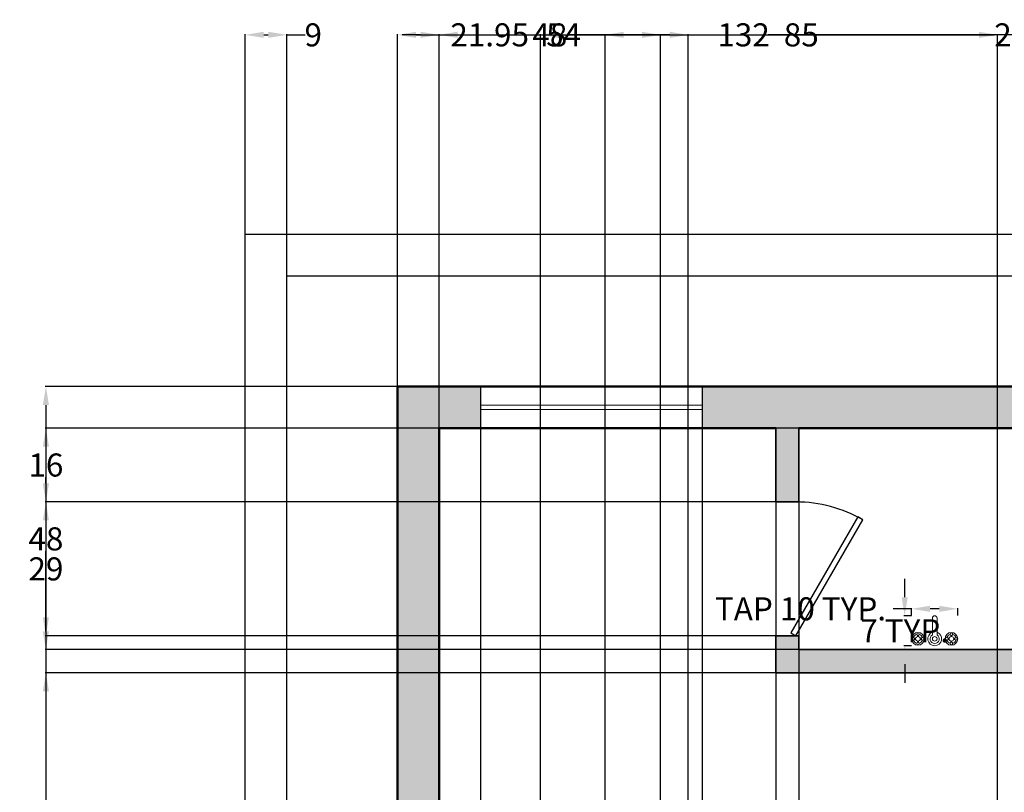
# Model space of a CAD drawing. Units: inches. Extents: x 882 to 1363, y 890 to 1847.
# Tile 8 of 9: x 901 to 1114, y 1680 to 1847. Entities that reach past the tile are written whole.
import ezdxf

# ---------------------------------------------------------------- set-up
doc = ezdxf.new("R2010")
doc.units = ezdxf.units.IN
doc.header["$MEASUREMENT"] = 0
for name, color, linetype, lineweight in [('A-ANNO-DIMS', 2, 'Continuous', 18), ('C-PROP', 7, 'Continuous', 25), ('doors', 3, 'Continuous', 25), ('inner wall', 50, 'Continuous', 35), ('outer wall', 40, 'Continuous', 50), ('sanitary', 231, 'Continuous', 18), ('windows', 226, 'Continuous', 18)]:
    doc.layers.add(name, color=color, linetype=linetype, lineweight=lineweight)
doc.layers.add('A-WALL-PATT', color=251, linetype='Continuous', lineweight=13, true_color=0x636466)
doc.styles.get("Standard").update_dxf_attribs({"font": 'arial.ttf'})
doc.dimstyles.get("Standard").update_dxf_attribs({"dimtxt": 5, "dimasz": 4, "dimexe": 0.18, "dimexo": 0.0625, "dimgap": 0.09, "dimtad": 0, "dimtih": 1, "dimtoh": 1, "dimdec": 1, "dimzin": 0, "dimdsep": 46, "dimlunit": 3, "dimtxsty": 'Standard', "dimcen": 0.09, "dimadec": 0, "dimazin": 0, "dimtfac": 1, "dimtdec": 1, "dimtofl": 0, "dimtmove": 0, "dimatfit": 3, "dimfxl": 1, "dimtolj": 1, "dimtzin": 0, "dimarcsym": 0})

# ---------------------------------------------------------------- blocks, each defined once
blk = doc.blocks.new('*U4')
for p, q in [((0, 0), (0, -6)), ((-40, 0), (-40, -6))]:
    blk.add_line(p, q)
blk.add_lwpolyline([(0, 0), (-34.64, 20), (-35.52, 18.48), (-0.88, -1.52)], close=True)
blk.add_arc((0, 0), 40, 150, 180)
blk = doc.blocks.new('Faucet - Bathroom top')
for p, q in [((-4.107, 0.125), (-4.375, 0.125)), ((-3.75, 0.4788), (-3.75, 0.75)), ((-3.5, 0.482), (-3.5, 0.75)), ((-3.1461, 0.125), (-2.875, 0.125)), ((3.143, 0.125), (2.875, 0.125)), ((3.5, 0.4788), (3.5, 0.75)), ((3.75, 0.482), (3.75, 0.75)), ((4.1039, 0.125), (4.375, 0.125)), ((-4.1039, -0.125), (-4.375, -0.125)), ((-3.75, -0.4821), (-3.75, -0.75)), ((-3.5, -0.4789), (-3.5, -0.75)), ((-3.143, -0.125), (-2.875, -0.125)), ((-0.5, -0.8639), (-0.5, -4.5)), ((0.5, -4.5), (0.5, -0.8631)), ((3.1461, -0.125), (2.875, -0.125)), ((3.5, -0.4821), (3.5, -0.75)), ((3.75, -0.4789), (3.75, -0.75)), ((4.107, -0.125), (4.375, -0.125))]:
    blk.add_line(p, q)
for centre, radius in [((-3.625, 0), 1.375), ((-4.625, 0), 0.2795), ((-3.625, 0), 0.5), ((-3.625, 1), 0.2795), ((-2.625, 0), 0.2795), ((0, 0), 0.5), ((3.625, 0), 1.375), ((2.625, 0), 0.2795), ((3.625, 0), 0.5), ((3.625, 1), 0.2795), ((4.625, 0), 0.2795), ((-3.625, -1), 0.2795), ((3.625, -1), 0.2795)]:
    blk.add_circle(centre, radius)
for centre, radius, start, end in [((-3.625, 0), 1, 105.2407, 164.2093), ((-3.625, 0), 1, 16.44125, 74.07887), ((0, 0), 1.5, 289.6514, 250.3603), ((0, 0), 1, 300.3431, 239.7554), ((3.625, 0), 1, 106.12, 164.0884), ((3.625, 0), 1, 16.23422, 73.90469), ((-3.625, 0), 1, 196.2342, 253.9047), ((-3.625, 0), 1, 286.12, 344.0884), ((3.625, 0), 1, 196.4413, 254.0789), ((3.625, 0), 1, 285.2407, 344.2093), ((0, -4.5), 0.5, 180, 0)]:
    blk.add_arc(centre, radius, start, end)
blk = doc.blocks.new('*D21')
at = {"layer": 'A-ANNO-DIMS', "color": 0, "lineweight": -2, "transparency": 16777216}
for p, q in [((1094.25, 1719.59), (1090.25, 1719.59)), ((1094.25, 1718.15), (1094.25, 1719.77)), ((1100.25, 1719.59), (1098.25, 1719.59)), ((1104.25, 1718.15), (1104.25, 1719.77))]:
    blk.add_line(p, q, dxfattribs=at)
at = {"layer": 'A-ANNO-DIMS', "color": 0, "transparency": 16777216}
for points in [[(1098.25, 1720.26), (1098.25, 1718.93), (1094.25, 1719.59)], [(1100.25, 1720.26), (1100.25, 1718.93), (1104.25, 1719.59)]]:
    blk.add_solid(points, dxfattribs=at)
at = {"layer": 'Defpoints', "color": 0, "transparency": 16777216}
for p in [(1094.25, 1719.59), (1094.25, 1718.09), (1104.25, 1718.09)]:
    blk.add_point(p, dxfattribs=at)
at = {"layer": 'A-ANNO-DIMS', "color": 0, "transparency": 16777216, "insert": (1070.17, 1719.59), "char_height": 5, "attachment_point": 5}
blk.add_mtext('\\A1;TAP 10 TYP.', dxfattribs=at)
blk = doc.blocks.new('*D22')
at = {"layer": 'A-ANNO-DIMS', "color": 0, "lineweight": -2, "transparency": 16777216}
for p, q in [((1092.75, 1722.09), (1092.75, 1726.09)), ((1094.19, 1718.09), (1092.57, 1718.09)), ((1094.19, 1711.59), (1092.57, 1711.59)), ((1092.75, 1707.59), (1092.75, 1703.59))]:
    blk.add_line(p, q, dxfattribs=at)
at = {"layer": 'A-ANNO-DIMS', "color": 0, "transparency": 16777216}
for points in [[(1092.09, 1722.09), (1093.42, 1722.09), (1092.75, 1718.09)], [(1092.09, 1707.59), (1093.42, 1707.59), (1092.75, 1711.59)]]:
    blk.add_solid(points, dxfattribs=at)
at = {"layer": 'Defpoints', "color": 0, "transparency": 16777216}
for p in [(1094.25, 1718.09), (1092.75, 1711.59), (1094.25, 1711.59)]:
    blk.add_point(p, dxfattribs=at)
at = {"layer": 'A-ANNO-DIMS', "color": 0, "transparency": 16777216, "insert": (1092.75, 1714.84), "char_height": 5, "attachment_point": 5}
blk.add_mtext('\\A1;7 TYP.', dxfattribs=at)
blk = doc.blocks.new('*D37')
at = {"layer": 'A-ANNO-DIMS', "color": 0, "lineweight": -2, "transparency": 16777216}
for p, q in [((982.78, 1767.75), (906.46, 1767.75)), ((906.64, 1763.75), (906.64, 1383.34)), ((906.64, 997.75), (906.64, 1378.16)), ((982.78, 993.75), (906.46, 993.75))]:
    blk.add_line(p, q, dxfattribs=at)
at = {"layer": 'A-ANNO-DIMS', "color": 0, "transparency": 16777216}
for points in [[(905.97, 1763.75), (907.3, 1763.75), (906.64, 1767.75)], [(905.97, 997.75), (907.3, 997.75), (906.64, 993.75)]]:
    blk.add_solid(points, dxfattribs=at)
at = {"layer": 'Defpoints', "color": 0, "transparency": 16777216}
for p in [(906.64, 1767.75), (982.84, 1767.75), (982.84, 993.75)]:
    blk.add_point(p, dxfattribs=at)
at = {"layer": 'A-ANNO-DIMS', "color": 0, "transparency": 16777216, "insert": (906.64, 1380.75), "char_height": 5, "attachment_point": 5}
blk.add_mtext('\\A1;774', dxfattribs=at)
blk = doc.blocks.new('*D38')
at = {"layer": 'A-ANNO-DIMS', "color": 0, "lineweight": -2, "transparency": 16777216}
for p, q in [((949.84, 1800.81), (949.84, 1844.13)), ((953.84, 1843.95), (954.84, 1843.95)), ((958.84, 1791.81), (958.84, 1844.13)), ((958.84, 1843.95), (962.84, 1843.95))]:
    blk.add_line(p, q, dxfattribs=at)
at = {"layer": 'A-ANNO-DIMS', "color": 0, "transparency": 16777216}
for points in [[(953.84, 1844.62), (953.84, 1843.29), (949.84, 1843.95)], [(954.84, 1844.62), (954.84, 1843.29), (958.84, 1843.95)]]:
    blk.add_solid(points, dxfattribs=at)
at = {"layer": 'Defpoints', "color": 0, "transparency": 16777216}
for p in [(958.84, 1843.95), (949.84, 1800.75), (958.84, 1791.75)]:
    blk.add_point(p, dxfattribs=at)
at = {"layer": 'A-ANNO-DIMS', "color": 0, "transparency": 16777216, "insert": (964.57, 1843.95), "char_height": 5, "attachment_point": 5}
blk.add_mtext('\\A1;9', dxfattribs=at)
blk = doc.blocks.new('*D39')
at = {"layer": 'A-ANNO-DIMS', "color": 0, "lineweight": -2, "transparency": 16777216}
for p, q in [((982.84, 1767.81), (982.84, 1844.13)), ((986.84, 1843.95), (1112.19, 1843.95)), ((1248.84, 1843.95), (1123.49, 1843.95)), ((1252.84, 1767.81), (1252.84, 1844.13))]:
    blk.add_line(p, q, dxfattribs=at)
at = {"layer": 'A-ANNO-DIMS', "color": 0, "transparency": 16777216}
for points in [[(986.84, 1844.62), (986.84, 1843.29), (982.84, 1843.95)], [(1248.84, 1844.62), (1248.84, 1843.29), (1252.84, 1843.95)]]:
    blk.add_solid(points, dxfattribs=at)
at = {"layer": 'Defpoints', "color": 0, "transparency": 16777216}
for p in [(1252.84, 1843.95), (982.84, 1767.75), (1252.84, 1767.75)]:
    blk.add_point(p, dxfattribs=at)
at = {"layer": 'A-ANNO-DIMS', "color": 0, "transparency": 16777216, "insert": (1117.84, 1843.95), "char_height": 5, "attachment_point": 5}
blk.add_mtext('\\A1;270', dxfattribs=at)
blk = doc.blocks.new('*D40')
at = {"layer": 'A-ANNO-DIMS', "color": 0, "lineweight": -2, "transparency": 16777216}
for p, q in [((991.84, 1758.69), (991.84, 893.37)), ((1064.84, 1758.69), (1064.84, 893.37)), ((995.84, 893.55), (1024.69, 893.55)), ((1060.84, 893.55), (1031.99, 893.55))]:
    blk.add_line(p, q, dxfattribs=at)
at = {"layer": 'A-ANNO-DIMS', "color": 0, "transparency": 16777216}
for points in [[(995.84, 894.21), (995.84, 892.88), (991.84, 893.55)], [(1060.84, 894.21), (1060.84, 892.88), (1064.84, 893.55)]]:
    blk.add_solid(points, dxfattribs=at)
at = {"layer": 'Defpoints', "color": 0, "transparency": 16777216}
for p in [(991.84, 1758.75), (1064.84, 1758.75), (1064.84, 893.55)]:
    blk.add_point(p, dxfattribs=at)
at = {"layer": 'A-ANNO-DIMS', "color": 0, "transparency": 16777216, "insert": (1028.34, 893.55), "char_height": 5, "attachment_point": 5}
blk.add_mtext('\\A1;73', dxfattribs=at)
blk = doc.blocks.new('*D41')
at = {"layer": 'A-ANNO-DIMS', "color": 0, "lineweight": -2, "transparency": 16777216}
for p, q in [((1069.84, 1758.69), (1069.84, 893.37)), ((1154.84, 1758.69), (1154.84, 893.37)), ((1073.84, 893.55), (1108.65, 893.55)), ((1150.84, 893.55), (1116.03, 893.55))]:
    blk.add_line(p, q, dxfattribs=at)
at = {"layer": 'A-ANNO-DIMS', "color": 0, "transparency": 16777216}
for points in [[(1073.84, 894.21), (1073.84, 892.88), (1069.84, 893.55)], [(1150.84, 894.21), (1150.84, 892.88), (1154.84, 893.55)]]:
    blk.add_solid(points, dxfattribs=at)
at = {"layer": 'Defpoints', "color": 0, "transparency": 16777216}
for p in [(1069.84, 1758.75), (1154.84, 1758.75), (1154.84, 893.55)]:
    blk.add_point(p, dxfattribs=at)
at = {"layer": 'A-ANNO-DIMS', "color": 0, "transparency": 16777216, "insert": (1112.34, 893.55), "char_height": 5, "attachment_point": 5}
blk.add_mtext('\\A1;85', dxfattribs=at)
blk = doc.blocks.new('*D43')
at = {"layer": 'A-ANNO-DIMS', "color": 0, "lineweight": -2, "transparency": 16777216}
for p, q in [((1243.78, 1758.75), (906.46, 1758.75)), ((906.64, 1754.75), (906.64, 1737.39)), ((906.64, 1714.75), (906.64, 1732.11)), ((1243.78, 1710.75), (906.46, 1710.75))]:
    blk.add_line(p, q, dxfattribs=at)
at = {"layer": 'A-ANNO-DIMS', "color": 0, "transparency": 16777216}
for points in [[(905.97, 1754.75), (907.3, 1754.75), (906.64, 1758.75)], [(905.97, 1714.75), (907.3, 1714.75), (906.64, 1710.75)]]:
    blk.add_solid(points, dxfattribs=at)
at = {"layer": 'Defpoints', "color": 0, "transparency": 16777216}
for p in [(1243.84, 1758.75), (906.64, 1710.75), (1243.84, 1710.75)]:
    blk.add_point(p, dxfattribs=at)
at = {"layer": 'A-ANNO-DIMS', "color": 0, "transparency": 16777216, "insert": (906.64, 1734.75), "char_height": 5, "attachment_point": 5}
blk.add_mtext('\\A1;48', dxfattribs=at)
blk = doc.blocks.new('*D44')
at = {"layer": 'A-ANNO-DIMS', "color": 0, "lineweight": -2, "transparency": 16777216}
for p, q in [((1243.78, 1705.75), (906.46, 1705.75)), ((906.64, 1701.75), (906.64, 1639.39)), ((906.64, 1571.75), (906.64, 1634.1)), ((1243.78, 1567.75), (906.46, 1567.75))]:
    blk.add_line(p, q, dxfattribs=at)
at = {"layer": 'A-ANNO-DIMS', "color": 0, "transparency": 16777216}
for points in [[(905.97, 1701.75), (907.3, 1701.75), (906.64, 1705.75)], [(905.97, 1571.75), (907.3, 1571.75), (906.64, 1567.75)]]:
    blk.add_solid(points, dxfattribs=at)
at = {"layer": 'Defpoints', "color": 0, "transparency": 16777216}
for p in [(1243.84, 1705.75), (906.64, 1567.75), (1243.84, 1567.75)]:
    blk.add_point(p, dxfattribs=at)
at = {"layer": 'A-ANNO-DIMS', "color": 0, "transparency": 16777216, "insert": (906.64, 1636.75), "char_height": 5, "attachment_point": 5}
blk.add_mtext('\\A1;138', dxfattribs=at)
blk = doc.blocks.new('*D46')
at = {"layer": 'A-ANNO-DIMS', "color": 0, "lineweight": -2, "transparency": 16777216}
for p, q in [((991.84, 1567.81), (991.84, 1844.13)), ((995.84, 1843.95), (1052.49, 1843.95)), ((1119.84, 1843.95), (1063.19, 1843.95)), ((1123.84, 1567.81), (1123.84, 1844.13))]:
    blk.add_line(p, q, dxfattribs=at)
at = {"layer": 'A-ANNO-DIMS', "color": 0, "transparency": 16777216}
for points in [[(995.84, 1844.62), (995.84, 1843.29), (991.84, 1843.95)], [(1119.84, 1844.62), (1119.84, 1843.29), (1123.84, 1843.95)]]:
    blk.add_solid(points, dxfattribs=at)
at = {"layer": 'Defpoints', "color": 0, "transparency": 16777216}
for p in [(1123.84, 1843.95), (991.84, 1567.75), (1123.84, 1567.75)]:
    blk.add_point(p, dxfattribs=at)
at = {"layer": 'A-ANNO-DIMS', "color": 0, "transparency": 16777216, "insert": (1057.84, 1843.95), "char_height": 5, "attachment_point": 5}
blk.add_mtext('\\A1;132', dxfattribs=at)
blk = doc.blocks.new('*D51')
at = {"layer": 'A-ANNO-DIMS', "color": 0, "lineweight": -2, "transparency": 16777216}
for p, q in [((982.84, 1767.69), (982.84, 893.37)), ((1000.84, 1767.69), (1000.84, 893.37)), ((986.84, 893.55), (996.84, 893.55)), ((1000.84, 893.55), (1004.84, 893.55))]:
    blk.add_line(p, q, dxfattribs=at)
at = {"layer": 'A-ANNO-DIMS', "color": 0, "transparency": 16777216}
for points in [[(986.84, 894.21), (986.84, 892.88), (982.84, 893.55)], [(996.84, 894.21), (996.84, 892.88), (1000.84, 893.55)]]:
    blk.add_solid(points, dxfattribs=at)
at = {"layer": 'Defpoints', "color": 0, "transparency": 16777216}
for p in [(982.84, 1767.75), (1000.84, 1767.75), (1000.84, 893.55)]:
    blk.add_point(p, dxfattribs=at)
at = {"layer": 'A-ANNO-DIMS', "color": 0, "transparency": 16777216, "insert": (1015.08, 893.55), "char_height": 5, "attachment_point": 5}
blk.add_mtext('\\A1;18.006', dxfattribs=at)
blk = doc.blocks.new('*D52')
at = {"layer": 'A-ANNO-DIMS', "color": 0, "lineweight": -2, "transparency": 16777216}
for p, q in [((1048.84, 1767.69), (1048.84, 893.37)), ((1118.86, 1767.69), (1118.86, 893.37)), ((1052.84, 893.55), (1075.83, 893.55)), ((1114.86, 893.55), (1091.87, 893.55))]:
    blk.add_line(p, q, dxfattribs=at)
at = {"layer": 'A-ANNO-DIMS', "color": 0, "transparency": 16777216}
for points in [[(1052.84, 894.21), (1052.84, 892.88), (1048.84, 893.55)], [(1114.86, 894.21), (1114.86, 892.88), (1118.86, 893.55)]]:
    blk.add_solid(points, dxfattribs=at)
at = {"layer": 'Defpoints', "color": 0, "transparency": 16777216}
for p in [(1048.84, 1767.75), (1118.86, 1767.75), (1118.86, 893.55)]:
    blk.add_point(p, dxfattribs=at)
at = {"layer": 'A-ANNO-DIMS', "color": 0, "transparency": 16777216, "insert": (1083.85, 893.55), "char_height": 5, "attachment_point": 5}
blk.add_mtext('\\A1;70.01', dxfattribs=at)
blk = doc.blocks.new('*D54')
at = {"layer": 'A-ANNO-DIMS', "color": 0, "lineweight": -2, "transparency": 16777216}
for p, q in [((1064.78, 1742.75), (906.46, 1742.75)), ((906.64, 1738.75), (906.64, 1730.89)), ((906.64, 1717.75), (906.64, 1725.61)), ((1064.78, 1713.75), (906.46, 1713.75))]:
    blk.add_line(p, q, dxfattribs=at)
at = {"layer": 'A-ANNO-DIMS', "color": 0, "transparency": 16777216}
for points in [[(905.97, 1738.75), (907.3, 1738.75), (906.64, 1742.75)], [(905.97, 1717.75), (907.3, 1717.75), (906.64, 1713.75)]]:
    blk.add_solid(points, dxfattribs=at)
at = {"layer": 'Defpoints', "color": 0, "transparency": 16777216}
for p in [(906.64, 1742.75), (1064.84, 1742.75), (1064.84, 1713.75)]:
    blk.add_point(p, dxfattribs=at)
at = {"layer": 'A-ANNO-DIMS', "color": 0, "transparency": 16777216, "insert": (906.64, 1728.25), "char_height": 5, "attachment_point": 5}
blk.add_mtext('\\A1;29', dxfattribs=at)
blk = doc.blocks.new('*D55')
at = {"layer": 'A-ANNO-DIMS', "color": 0, "lineweight": -2, "transparency": 16777216}
for p, q in [((1064.78, 1758.75), (906.46, 1758.75)), ((906.64, 1754.75), (906.64, 1753.39)), ((906.64, 1746.75), (906.64, 1748.11)), ((1064.78, 1742.75), (906.46, 1742.75))]:
    blk.add_line(p, q, dxfattribs=at)
at = {"layer": 'A-ANNO-DIMS', "color": 0, "transparency": 16777216}
for points in [[(905.97, 1754.75), (907.3, 1754.75), (906.64, 1758.75)], [(905.97, 1746.75), (907.3, 1746.75), (906.64, 1742.75)]]:
    blk.add_solid(points, dxfattribs=at)
at = {"layer": 'Defpoints', "color": 0, "transparency": 16777216}
for p in [(1064.84, 1758.75), (906.64, 1742.75), (1064.84, 1742.75)]:
    blk.add_point(p, dxfattribs=at)
at = {"layer": 'A-ANNO-DIMS', "color": 0, "transparency": 16777216, "insert": (906.64, 1750.75), "char_height": 5, "attachment_point": 5}
blk.add_mtext('\\A1;16', dxfattribs=at)
blk = doc.blocks.new('*D57')
at = {"layer": 'A-ANNO-DIMS', "color": 0, "lineweight": -2, "transparency": 16777216}
for p, q in [((991.84, 1478.81), (991.84, 1844.13)), ((995.84, 1843.95), (1015.18, 1843.95)), ((1041.84, 1843.95), (1022.5, 1843.95)), ((1045.84, 1478.81), (1045.84, 1844.13))]:
    blk.add_line(p, q, dxfattribs=at)
at = {"layer": 'A-ANNO-DIMS', "color": 0, "transparency": 16777216}
for points in [[(995.84, 1844.62), (995.84, 1843.29), (991.84, 1843.95)], [(1041.84, 1844.62), (1041.84, 1843.29), (1045.84, 1843.95)]]:
    blk.add_solid(points, dxfattribs=at)
at = {"layer": 'Defpoints', "color": 0, "transparency": 16777216}
for p in [(1045.84, 1843.95), (991.84, 1478.75), (1045.84, 1478.75)]:
    blk.add_point(p, dxfattribs=at)
at = {"layer": 'A-ANNO-DIMS', "color": 0, "transparency": 16777216, "insert": (1018.84, 1843.95), "char_height": 5, "attachment_point": 5}
blk.add_mtext('\\A1;54', dxfattribs=at)
blk = doc.blocks.new('*D68')
at = {"layer": 'A-ANNO-DIMS', "color": 0, "lineweight": -2, "transparency": 16777216}
for p, q in [((1027.84, 1142.81), (1027.84, 1844.13)), ((1031.84, 1843.95), (1066.65, 1843.95)), ((1108.84, 1843.95), (1074.03, 1843.95)), ((1112.84, 1142.81), (1112.84, 1844.13))]:
    blk.add_line(p, q, dxfattribs=at)
at = {"layer": 'A-ANNO-DIMS', "color": 0, "transparency": 16777216}
for points in [[(1031.84, 1844.62), (1031.84, 1843.29), (1027.84, 1843.95)], [(1108.84, 1844.62), (1108.84, 1843.29), (1112.84, 1843.95)]]:
    blk.add_solid(points, dxfattribs=at)
at = {"layer": 'Defpoints', "color": 0, "transparency": 16777216}
for p in [(1112.84, 1843.95), (1027.84, 1142.75), (1112.84, 1142.75)]:
    blk.add_point(p, dxfattribs=at)
at = {"layer": 'A-ANNO-DIMS', "color": 0, "transparency": 16777216, "insert": (1070.34, 1843.95), "char_height": 5, "attachment_point": 5}
blk.add_mtext('\\A1;85', dxfattribs=at)
blk = doc.blocks.new('*D74')
at = {"layer": 'A-ANNO-DIMS', "color": 0, "lineweight": -2, "transparency": 16777216}
for p, q in [((991.84, 1002.81), (991.84, 1844.13)), ((995.84, 1843.95), (1012.06, 1843.95)), ((1035.84, 1843.95), (1019.62, 1843.95)), ((1039.84, 1002.81), (1039.84, 1844.13))]:
    blk.add_line(p, q, dxfattribs=at)
at = {"layer": 'A-ANNO-DIMS', "color": 0, "transparency": 16777216}
for points in [[(995.84, 1844.62), (995.84, 1843.29), (991.84, 1843.95)], [(1035.84, 1844.62), (1035.84, 1843.29), (1039.84, 1843.95)]]:
    blk.add_solid(points, dxfattribs=at)
at = {"layer": 'Defpoints', "color": 0, "transparency": 16777216}
for p in [(1039.84, 1843.95), (991.84, 1002.75), (1039.84, 1002.75)]:
    blk.add_point(p, dxfattribs=at)
at = {"layer": 'A-ANNO-DIMS', "color": 0, "transparency": 16777216, "insert": (1015.84, 1843.95), "char_height": 5, "attachment_point": 5}
blk.add_mtext('\\A1;48', dxfattribs=at)
blk = doc.blocks.new('*D93')
at = {"layer": 'A-ANNO-DIMS', "color": 0, "lineweight": -2, "transparency": 16777216}
for p, q in [((987.84, 1843.95), (983.84, 1843.95)), ((991.84, 1337.4), (991.84, 1844.13)), ((1013.79, 1306.45), (1013.79, 1844.13)), ((1017.79, 1843.95), (1021.79, 1843.95))]:
    blk.add_line(p, q, dxfattribs=at)
at = {"layer": 'A-ANNO-DIMS', "color": 0, "transparency": 16777216}
for points in [[(987.84, 1844.62), (987.84, 1843.29), (991.84, 1843.95)], [(1017.79, 1844.62), (1017.79, 1843.29), (1013.79, 1843.95)]]:
    blk.add_solid(points, dxfattribs=at)
at = {"layer": 'Defpoints', "color": 0, "transparency": 16777216}
for p in [(1013.79, 1843.95), (991.84, 1337.33), (1013.79, 1306.39)]:
    blk.add_point(p, dxfattribs=at)
at = {"layer": 'A-ANNO-DIMS', "color": 0, "transparency": 16777216, "insert": (1002.81, 1843.95), "char_height": 5, "attachment_point": 5}
blk.add_mtext('\\A1;21.95', dxfattribs=at)

msp = doc.modelspace()

# ---------------------------------------------------------------- hatches: boundary and pattern name
at = {"layer": 'A-WALL-PATT'}
h = msp.add_hatch(color=256, dxfattribs=at)
h.dxf.hatch_style = 1
h.paths.add_polyline_path([(1050.8388, 1481.7495), (1050.8388, 1478.7495), (1084.8388, 1478.7495), (1084.8388, 1473.7495), (991.8388, 1473.7495), (991.8388, 1361.0778), (982.8388, 1361.0778), (982.8388, 1556.1531), (991.8388, 1556.1531), (991.8388, 1478.7495), (1045.8388, 1478.7495), (1045.8388, 1481.7479), (1045.4161, 1481.7477), (1030.9055, 1506.8563), (1032.004, 1507.4911), (1046.5146, 1482.3825), (1045.4161, 1481.7477), (1045.8388, 1481.7479), (1045.8388, 1481.7495)])
h.paths.add_polyline_path([(1128.8388, 1478.7495), (1120.8388, 1478.7495), (1120.8388, 1473.7495), (1123.8388, 1473.7495), (1123.8388, 1353.7495), (991.8388, 1353.7495), (991.8388, 1361.0778), (982.8388, 1361.0778), (982.8388, 1337.3333), (991.8388, 1337.3333), (991.8388, 1348.7495), (1128.8388, 1348.7495)])
h.paths.add_polyline_path([(1118.8585, 1767.7495), (1048.8447, 1767.7495), (1048.8447, 1758.7495), (1064.8388, 1758.7495), (1069.8388, 1758.7495), (1118.8585, 1758.7495)])
h.paths.add_polyline_path([(1171.4129, 1767.7495), (1142.8585, 1767.7495), (1142.8585, 1758.7495), (1154.8388, 1758.7495), (1154.8388, 1710.7495), (1069.8388, 1710.7495), (1069.8388, 1713.7495), (1064.8388, 1713.7495), (1064.8388, 1705.7495), (1123.8388, 1705.7495), (1123.8388, 1567.7495), (1120.8388, 1567.7495), (1120.8388, 1562.7495), (1123.8388, 1562.7495), (1211.8388, 1562.7495), (1211.8388, 1567.7495), (1128.8388, 1567.7495), (1128.8388, 1705.7495), (1211.8388, 1705.7495), (1211.8388, 1710.7495), (1159.8388, 1710.7495), (1159.8388, 1758.7495), (1171.4129, 1758.7495)])
h.paths.add_polyline_path([(1252.8388, 1767.7495), (1195.4129, 1767.7495), (1195.4129, 1758.7495), (1243.8388, 1758.7495), (1243.8388, 1710.7495), (1240.8388, 1710.7495), (1240.8388, 1706.4648), (1240.8388, 1705.7495), (1243.8388, 1705.7495), (1243.8388, 1673.1735), (1252.8388, 1673.1735)])
h.paths.add_polyline_path([(1252.8388, 1625.1735), (1243.8388, 1625.1735), (1243.8388, 1567.7495), (1240.8388, 1567.7495), (1240.8388, 1562.7495), (1243.8388, 1562.7495), (1243.8388, 1546.029), (1252.8388, 1546.029)])
h.paths.add_polyline_path([(1252.8388, 1498.029), (1243.8388, 1498.029), (1243.8388, 1391.1399), (1252.8388, 1391.1399)])
h.paths.add_polyline_path([(1252.8388, 1179.8561), (1243.8388, 1179.8561), (1243.8388, 1149.7495), (1219.8388, 1149.7495), (1219.8388, 1145.3111), (1219.8388, 1144.7495), (1252.8388, 1144.7495)])
h.paths.add_polyline_path([(1252.8388, 1277.7495), (1243.8388, 1277.7495), (1243.8388, 1274.7495), (1219.8388, 1274.7495), (1219.8388, 1269.7495), (1243.8388, 1269.7495), (1243.8388, 1227.8561), (1252.8388, 1227.8561)])
h.paths.add_polyline_path([(1252.8388, 1343.1399), (1243.8388, 1343.1399), (1243.8388, 1313.7495), (1248.3388, 1313.7495), (1252.8388, 1313.7495)])
h.paths.add_polyline_path([(1146.8388, 1274.7495), (1112.8388, 1274.7495), (1112.8388, 1106.7495), (1106.7761, 1106.7495), (1106.7761, 1101.7495), (1117.8388, 1101.7495), (1117.8388, 1144.7495), (1159.8388, 1144.7495), (1159.8388, 1149.7495), (1117.8388, 1149.7495), (1117.8388, 1269.7495), (1146.8388, 1269.7495)])
h = msp.add_hatch(color=256, dxfattribs=at)
h.dxf.hatch_style = 1
h.paths.add_polyline_path([(1000.8447, 1767.7495), (993.3979, 1767.7495), (991.8388, 1758.7495), (1000.8447, 1758.7495)])
h.paths.add_polyline_path([(991.8388, 1654.8981), (982.8388, 1654.3544), (982.8388, 1595.0521), (991.8388, 1594.8981)])
h.paths.add_polyline_path([(991.8388, 1594.8981), (982.8388, 1595.0521), (982.8388, 1559.7196), (991.8388, 1562.7495), (991.8388, 1567.7495)])
h.paths.add_polyline_path([(991.8388, 1562.7495), (982.8388, 1559.7196), (982.8388, 1556.1531), (991.8388, 1556.1531)])
h.paths.add_polyline_path([(991.8388, 1289.3333), (982.8388, 1289.3333), (982.8388, 1265.8272), (991.8388, 1265.8272)])
h.paths.add_polyline_path([(1058.7761, 1106.7495), (991.8388, 1106.7495), (982.8388, 1107.8066), (982.8388, 1101.3439), (991.8388, 1101.7495), (1058.7761, 1101.7495)])
h = msp.add_hatch(color=256, dxfattribs=at)
h.dxf.hatch_style = 1
h.paths.add_polyline_path([(993.3979, 1767.7495), (982.8388, 1767.7495), (982.8388, 1752.9363), (991.8388, 1758.7495)])
h.paths.add_polyline_path([(991.8388, 1758.7495), (982.8388, 1752.9363), (982.8388, 1654.3544), (991.8388, 1654.8981), (991.8388, 1710.7495)])
h.paths.add_polyline_path([(1050.8388, 1562.7495), (1084.8388, 1562.7495), (1084.8388, 1567.7495), (991.8388, 1567.7495), (991.8388, 1562.7495), (1045.8388, 1562.7495), (1045.8388, 1510.7495), (1050.8388, 1510.7495)])
h = msp.add_hatch(color=256, dxfattribs=at)
h.dxf.hatch_style = 1
h.paths.add_polyline_path([(1069.8388, 1758.7495), (1118.8585, 1758.7495), (1118.8585, 1767.7495), (1048.8447, 1767.7495), (1048.8447, 1758.7495), (1064.8388, 1758.7495), (1064.8388, 1742.7495), (1069.8388, 1742.7495)])

# ---------------------------------------------------------------- linework, layer by layer
at = {"layer": 'C-PROP'}
for points in [[(949.8388, 1800.7495), (1309.8388, 1800.7495), (1309.8388, 936.7495), (949.8388, 936.7495)], [(958.8388, 1791.7495), (1300.8388, 1791.7495), (1300.8388, 945.7495), (958.8388, 945.7495)]]:
    msp.add_lwpolyline(points, close=True, dxfattribs=at)
at = {"layer": 'inner wall'}
for p, q in [((1064.8388, 1758.7495), (1064.8388, 1742.7495)), ((1069.8388, 1758.7495), (1069.8388, 1742.7495)), ((1064.8388, 1742.7495), (1069.8388, 1742.7495)), ((1064.8388, 1713.7495), (1069.8388, 1713.7495)), ((1064.8388, 1713.7495), (1064.8388, 1705.7495)), ((1069.8388, 1713.7495), (1069.8388, 1710.7495)), ((1069.8388, 1710.7495), (1154.8388, 1710.7495)), ((1064.8388, 1705.7495), (1123.8388, 1705.7495))]:
    msp.add_line(p, q, dxfattribs=at)
at = {"layer": 'outer wall'}
for p, q in [((982.8388, 993.7495), (982.8388, 1767.7495)), ((982.8388, 1767.7495), (1252.8388, 1767.7495)), ((991.8388, 1758.7495), (1064.8388, 1758.7495)), ((991.8388, 1710.7495), (991.8388, 1758.7495)), ((1069.8388, 1758.7495), (1154.8388, 1758.7495)), ((991.8388, 1567.7495), (991.8388, 1710.7495))]:
    msp.add_line(p, q, dxfattribs=at)
at = {"layer": 'windows'}
for p, q in [((1000.8447, 1763.7495), (1048.8447, 1763.7495)), ((1000.8447, 1762.7495), (1048.8447, 1762.7495))]:
    msp.add_line(p, q, dxfattribs=at)
msp.add_lwpolyline([(1048.8447, 1767.7495), (1048.8447, 1758.7495), (1000.8447, 1758.7495), (1000.8447, 1767.7495)], close=True, dxfattribs=at)

# ---------------------------------------------------------------- block references
at = {"layer": 'doors', "xscale": 0.7249999999999942, "yscale": 0.7249999999999942, "zscale": 0.7249999999999942, "rotation": 270.0000000000005}
msp.add_blockref('*U4', (1069.1888, 1713.7495), dxfattribs=at)
at = {"layer": 'sanitary', "rotation": 180}
msp.add_blockref('Faucet - Bathroom top', (1099.2523, 1713.0924), dxfattribs=at)

# ---------------------------------------------------------------- dimensions: what is measured, and where the dimension line sits
at = {"layer": 'A-ANNO-DIMS'}
for base, p1, p2, override, picture, middle in [((958.8388, 1843.953), (949.8388, 1800.7495), (958.8388, 1791.7495), {"dimdec": 0, "dimlfac": 1, "dimrnd": 0, "dimzin": 0, "dimdsep": 46, "dimlunit": 2}, '*D38', (964.5728, 1843.953)), ((1252.8388, 1843.953), (982.8388, 1767.7495), (1252.8388, 1767.7495), {"dimdec": 0, "dimlfac": 1, "dimrnd": 0, "dimzin": 0, "dimdsep": 46, "dimlunit": 2}, '*D39', (1117.8388, 1843.953)), ((1013.7874, 1843.953), (991.8388, 1337.3333), (1013.7874, 1306.3919), {"dimdec": 2, "dimlfac": 1, "dimrnd": 0, "dimzin": 0, "dimdsep": 46, "dimlunit": 2}, '*D93', (1002.8131, 1843.953)), ((1123.8388, 1843.953), (991.8388, 1567.7495), (1123.8388, 1567.7495), {"dimdec": 0, "dimlfac": 1, "dimrnd": 0, "dimzin": 0, "dimdsep": 46, "dimlunit": 2}, '*D46', (1057.8388, 1843.953)), ((1045.8388, 1843.953), (991.8388, 1478.7495), (1045.8388, 1478.7495), {"dimdec": 0, "dimlfac": 1, "dimrnd": 0, "dimzin": 0, "dimdsep": 46, "dimlunit": 2}, '*D57', (1018.8388, 1843.953)), ((1039.8388, 1843.953), (991.8388, 1002.7495), (1039.8388, 1002.7495), {"dimdec": 0, "dimlfac": 1, "dimrnd": 0, "dimzin": 0, "dimdsep": 46, "dimlunit": 2}, '*D74', (1015.8388, 1843.953)), ((1112.8388, 1843.953), (1027.8388, 1142.7495), (1112.8388, 1142.7495), {"dimdec": 0, "dimlfac": 1, "dimrnd": 0, "dimzin": 0, "dimdsep": 46, "dimlunit": 2}, '*D68', (1070.3388, 1843.953)), ((1000.8447, 893.546), (982.8388, 1767.7495), (1000.8447, 1767.7495), {"dimdec": 3, "dimlfac": 1, "dimrnd": 0, "dimzin": 0, "dimdsep": 46, "dimlunit": 2}, '*D51', (1015.0762, 893.546)), ((1118.8585, 893.546), (1048.8447, 1767.7495), (1118.8585, 1767.7495), {"dimdec": 2, "dimlfac": 1, "dimrnd": 0, "dimzin": 0, "dimdsep": 46, "dimlunit": 2}, '*D52', (1083.8516, 893.546)), ((1064.8388, 893.546), (991.8388, 1758.7495), (1064.8388, 1758.7495), {"dimdec": 0, "dimlfac": 1, "dimrnd": 0, "dimzin": 0, "dimdsep": 46, "dimlunit": 2}, '*D40', (1028.3388, 893.546)), ((1154.8388, 893.546), (1069.8388, 1758.7495), (1154.8388, 1758.7495), {"dimdec": 0, "dimlfac": 1, "dimrnd": 0, "dimzin": 0, "dimdsep": 46, "dimlunit": 2}, '*D41', (1112.3388, 893.546))]:
    dim = msp.add_linear_dim(base=base, p1=p1, p2=p2, dimstyle='Standard', override=override, dxfattribs=at)
    dim.commit()
    dim.dimension.update_dxf_attribs({"geometry": picture, "text_midpoint": middle})
for base, p1, p2, picture, middle in [((906.6353, 1767.7495), (982.8388, 993.7495), (982.8388, 1767.7495), '*D37', (906.6353, 1380.7495)), ((906.6353, 1710.7495), (1243.8388, 1758.7495), (1243.8388, 1710.7495), '*D43', (906.6353, 1734.7495)), ((906.6353, 1742.7495), (1064.8388, 1758.7495), (1064.8388, 1742.7495), '*D55', (906.6353, 1750.7495)), ((906.6353, 1742.7495), (1064.8388, 1713.7495), (1064.8388, 1742.7495), '*D54', (906.6353, 1728.2495)), ((906.6353, 1567.7495), (1243.8388, 1705.7495), (1243.8388, 1567.7495), '*D44', (906.6353, 1636.7495))]:
    dim = msp.add_linear_dim(base=base, p1=p1, p2=p2, angle=90, dimstyle='Standard', override={"dimdec": 0, "dimlfac": 1, "dimrnd": 0, "dimzin": 0, "dimdsep": 46, "dimlunit": 2}, dxfattribs=at)
    dim.commit()
    dim.dimension.update_dxf_attribs({"geometry": picture, "text_midpoint": middle})
for base, p1, p2, angle, text, picture, middle in [((1094.2523, 1719.5924), (1104.2523, 1718.0924), (1094.2523, 1718.0924), 180, 'TAP <> TYP.', '*D21', (1070.1674, 1719.5924)), ((1092.7523, 1711.5923), (1094.2523, 1718.0924), (1094.2523, 1711.5923), 270, '<> TYP.', '*D22', (1092.7523, 1714.8423))]:
    dim = msp.add_linear_dim(base=base, p1=p1, p2=p2, angle=angle, text=text, dimstyle='Standard', override={"dimdec": 0, "dimlfac": 1, "dimrnd": 0, "dimzin": 0, "dimdsep": 46, "dimlunit": 2}, dxfattribs=at)
    dim.commit()
    dim.dimension.update_dxf_attribs({"geometry": picture, "text_midpoint": middle})

doc.saveas('drawing.dxf')
